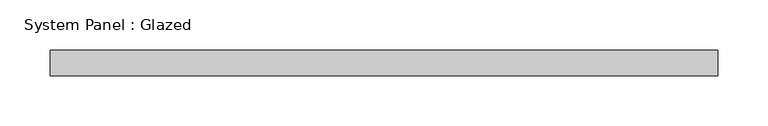
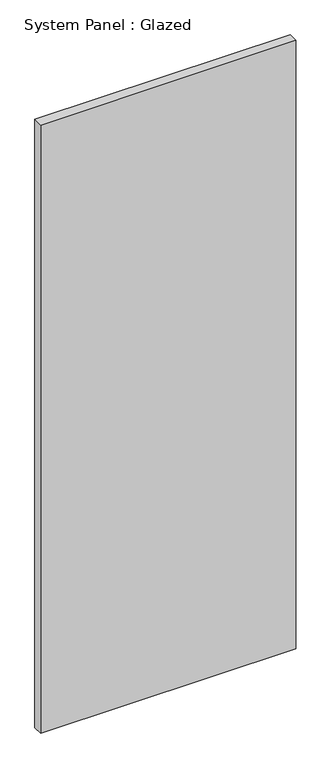
"""IFC4 building model written with IfcOpenShell, lengths in millimetres: plate geometry, System Panel : Glazed."""

from ifc_helpers import new_model, si_unit, origin, origin_with_axes, place, context, project, spatial, polyline, outline, extrude, source, transform, mapped, element, save


def system_panel_glazed_aca50f87(model_context):
    return source(origin(), model_context, "Body", "SweptSolid", [
        extrude(outline(polyline([(333.375, 19.05), (-333.375, 19.05), (-333.375, 44.45), (333.375, 44.45), (333.375, 19.05)])), origin_with_axes(), (0.0, 0.0, 1.0), 1678.4265918),
    ])


if __name__ == "__main__":
    model = new_model("IFC4")
    model_context = context("Model", 3, world=origin())
    ifc_project = project(units=[si_unit("LENGTHUNIT", "METRE", prefix="MILLI")], contexts=[model_context])
    site = spatial("IfcSite", under=ifc_project)
    building = spatial("IfcBuilding", under=site)
    placement = place(None, origin())
    system_panel_glazed_shape = system_panel_glazed_aca50f87(model_context)
    element("IfcPlate", 1, ObjectType="System Panel : Glazed", at=placement, inside=building, context=model_context, shape_type="MappedRepresentation", body=[
        mapped(system_panel_glazed_shape, transform((0.0, 0.0, 0.0), x_axis=(1.0, 0.0, 0.0), y_axis=(0.0, 1.0, 0.0), z_axis=(0.0, 0.0, 1.0))),
    ])
    save(model, "model.ifc")

# Revit data of these elements
# Type "System Panel : Glazed"
#   Construction Type Id = "GSP4R"
#   Analytic Construction = "1/8 in Pilkington single glazing"
#   Visual Light Transmittance = 0.9
#   Solar Heat Gain Coefficient = 0.86
#   Heat Transfer Coefficient (U) = 1.18115 BTU/(h·ft²·°F)
#   Define Thermal Properties by = 1
# Element 1 (IfcPlate, "System Panel : Glazed")
#   Materials on its faces: "Glass"
# Materials
#   "Glass": class "Glass", colour RGB 0 128 192, transparency 0.75, Description = "Soda Lime Glass", Cost = 0
